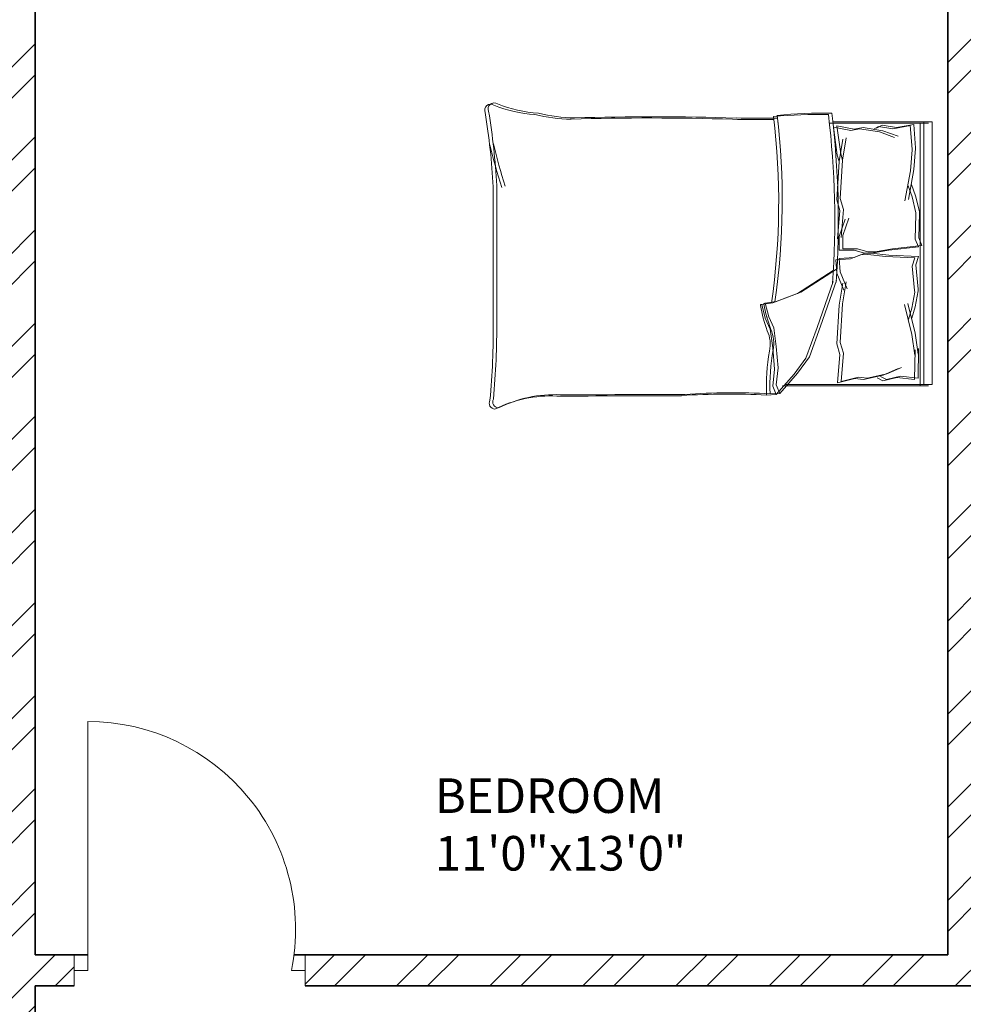
# Model space of a CAD drawing. Units: inches. Extents: x 1962 to 2771, y 1245 to 2660.
# Tile 111 of 114: x 2374 to 2510, y 2304 to 2447. Entities that reach past the tile are written whole.
import ezdxf

# ---------------------------------------------------------------- set-up
doc = ezdxf.new("R2010")
doc.units = ezdxf.units.IN
for name, color, linetype, lineweight in [('A-ANNO-DIMS', 2, 'Continuous', 18), ('A-AREA-IDEN', 7, 'Continuous', 18), ('A-DOOR', 3, 'Continuous', 18), ('A-FURN', 8, 'Continuous', 13), ('A-WALL', 7, 'Continuous', 35), ('A-WALL-PATT', 252, 'Continuous', 13)]:
    doc.layers.add(name, color=color, linetype=linetype, lineweight=lineweight)
doc.styles.get("Standard").update_dxf_attribs({"font": 'arial.ttf'})
doc.dimstyles.get("Standard").update_dxf_attribs({"dimtxt": 0.18, "dimasz": 0.18, "dimexe": 0.18, "dimexo": 0.0625, "dimgap": 0.09, "dimtad": 0, "dimtih": 1, "dimtoh": 1, "dimdec": 4, "dimzin": 0, "dimdsep": 46, "dimtxsty": 'Standard', "dimcen": 0.09, "dimadec": 0, "dimazin": 0, "dimtfac": 1, "dimtdec": 4, "dimtofl": 0, "dimtmove": 0, "dimatfit": 3, "dimfxl": 1, "dimtolj": 1, "dimtzin": 0, "dimarcsym": 0})

# ---------------------------------------------------------------- blocks, each defined once
blk = doc.blocks.new('BED-PLAN')
for p, q in [((22.05, 42.03), (19.47, 39.08)), ((22.05, 42.02), (19.47, 39.08)), ((22.56, 42.21), (19.98, 39.26)), ((22.56, 42.21), (19.98, 39.26)), ((23.44, 42.09), (22.05, 42.03, 3.08)), ((23.44, 42.09), (22.05, 42.02, 3.08)), ((22.55, 40.8), (22.05, 42.03)), ((22.55, 40.8), (22.05, 42.02)), ((23.95, 42.27), (22.56, 42.21, 3.08)), ((23.95, 42.27), (22.56, 42.21, 3.08)), ((23.06, 40.98), (22.56, 42.21)), ((23.06, 40.98), (22.56, 42.21)), ((0, 40.75), (21.15, 40.75)), ((0, 40.75), (21.15, 40.75)), ((0, 2.76), (0, 40.75)), ((0.51, 40.93), (21.66, 40.93)), ((0.51, 40.93), (21.66, 40.93)), ((1.22, 2.76), (1.22, 40.75)), ((1.22, 2.76), (1.22, 40.75)), ((1.73, 2.95), (1.73, 40.93)), ((1.73, 2.95), (1.73, 40.93)), ((2.54, 40.02), (2.46, 35.72)), ((2.54, 40.02), (2.46, 35.72)), ((2.54, 40.02), (5.09, 39.72)), ((2.54, 40.02), (5.09, 39.72)), ((4.58, 39.53), (6.63, 40.01)), ((4.58, 39.53), (6.63, 40.01)), ((5.09, 39.72), (7.14, 40.19)), ((5.09, 39.72), (7.14, 40.19)), ((6.63, 40.01), (7.46, 39.6)), ((6.63, 40.01), (7.46, 39.6)), ((9.91, 40.02), (7.07, 39.38)), ((9.91, 40.02), (7.07, 39.38)), ((7.14, 40.19), (7.97, 39.78)), ((7.14, 40.19), (7.97, 39.78)), ((11.19, 39.87), (9.91, 40.02)), ((11.19, 39.87), (9.91, 40.02)), ((13.17, 40.3), (10.68, 39.68)), ((13.17, 40.3), (10.68, 39.68)), ((13.68, 40.48), (11.19, 39.87)), ((13.68, 40.48), (11.19, 39.87)), ((12.85, 36.22), (13.17, 40.3)), ((12.85, 36.22), (13.17, 40.3)), ((13.36, 36.4), (13.68, 40.48)), ((13.36, 36.4), (13.68, 40.48)), ((22.3, 38.34), (22.55, 40.8)), ((22.3, 38.34), (22.55, 40.8)), ((22.81, 38.52), (23.06, 40.98)), ((22.81, 38.52), (23.06, 40.98)), ((2.03, 39.83), (1.96, 35.54)), ((2.03, 39.83), (1.96, 35.54)), ((2.03, 39.83), (4.58, 39.53)), ((2.03, 39.83), (4.58, 39.53)), ((6.56, 39.2), (4.43, 38.26)), ((6.56, 39.2), (4.43, 38.26)), ((7.07, 39.38), (4.94, 38.44)), ((7.07, 39.38), (4.94, 38.44)), ((9.4, 39.83), (6.56, 39.2)), ((9.4, 39.83), (6.56, 39.2)), ((10.68, 39.68), (9.4, 39.83)), ((10.68, 39.68), (9.4, 39.83)), ((19.47, 39.08), (17.75, 36.74)), ((19.47, 39.08), (17.75, 36.74)), ((19.98, 39.26), (18.26, 36.92)), ((19.98, 39.26), (18.26, 36.92)), ((23.06, 35.45), (22.81, 38.52)), ((23.06, 35.44), (22.81, 38.52)), ((22.55, 35.26), (22.3, 38.34)), ((22.55, 35.26), (22.3, 38.34)), ((1.96, 35.54), (2.02, 36.34)), ((1.96, 35.54), (2.02, 36.34)), ((2.02, 36.34), (2.44, 33.32)), ((2.02, 36.34), (2.44, 33.32)), ((2.46, 35.72), (2.53, 36.52)), ((2.46, 35.72), (2.53, 36.52)), ((2.53, 36.52), (2.95, 33.5)), ((2.53, 36.52), (2.95, 33.5)), ((13.3, 34.66), (12.85, 36.22)), ((13.3, 34.66), (12.85, 36.22)), ((13.8, 34.84), (13.36, 36.4)), ((13.8, 34.84), (13.36, 36.4)), ((17.75, 36.74), (16.15, 32.31)), ((17.75, 36.74), (16.15, 32.31)), ((18.26, 36.92), (16.66, 32.49)), ((18.26, 36.92), (16.66, 32.49)), ((12.95, 29.09), (13.3, 34.66)), ((12.95, 29.09), (13.3, 34.66)), ((13.46, 29.27), (13.8, 34.84)), ((13.46, 29.27), (13.8, 34.84)), ((22.92, 32.56), (22.55, 35.26)), ((22.92, 32.55), (22.55, 35.26)), ((23.42, 32.74), (23.06, 35.45)), ((23.42, 32.74), (23.06, 35.44)), ((2.44, 33.32), (3.52, 29.01)), ((2.44, 33.32), (3.52, 29.01)), ((2.95, 33.5), (4.02, 29.19)), ((2.95, 33.5), (4.02, 29.19)), ((3.43, 31.34), (2.96, 29.7)), ((3.43, 31.34), (2.96, 29.7)), ((16.15, 32.31), (13.82, 25.68)), ((16.15, 32.31), (13.82, 25.68)), ((16.66, 32.49), (14.33, 25.86)), ((16.66, 32.49), (14.33, 25.86)), ((23.65, 30.95), (22.92, 32.56)), ((23.65, 30.95), (22.92, 32.55)), ((24.16, 31.14), (23.42, 32.74)), ((24.16, 31.14), (23.42, 32.74)), ((62.99, 11.98), (62.99, 31.54)), ((62.99, 11.97), (62.99, 31.54)), ((63.5, 12.16), (63.5, 31.72)), ((63.5, 12.16), (63.5, 31.72)), ((2.92, 31.16), (2.45, 29.52)), ((2.92, 31.16), (2.45, 29.52)), ((24.15, 28.99), (23.65, 30.95)), ((24.15, 28.98), (23.65, 30.95)), ((24.65, 29.17), (24.16, 31.14)), ((24.65, 29.17), (24.16, 31.14)), ((2.45, 29.52), (2.02, 27.19)), ((2.45, 29.52), (2.02, 27.19)), ((2.96, 29.7), (2.52, 27.37)), ((2.96, 29.7), (2.52, 27.37)), ((12.42, 25.89), (12.95, 29.09)), ((12.42, 25.89), (12.95, 29.09)), ((12.93, 26.07), (13.46, 29.27)), ((12.93, 26.07), (13.46, 29.27)), ((18.98, 27.38), (22.55, 28.74)), ((18.98, 27.38), (22.55, 28.74)), ((19.49, 27.57), (23.06, 28.92)), ((19.49, 27.57), (23.06, 28.92)), ((22.55, 28.74), (24.15, 28.99)), ((22.55, 28.74), (24.15, 28.98)), ((23.06, 28.92), (24.65, 29.17)), ((23.06, 28.92), (24.65, 29.17)), ((2.02, 27.19), (2.03, 26.94)), ((2.02, 27.19), (2.03, 26.93)), ((2.52, 27.37), (2.54, 27.12)), ((2.52, 27.37), (2.54, 27.12)), ((2.54, 27.12), (2.88, 23.6)), ((2.54, 27.12), (2.88, 23.6)), ((13.82, 24.05), (18.98, 27.38)), ((13.82, 24.05), (18.98, 27.38)), ((14.33, 24.24), (19.49, 27.57)), ((14.33, 24.24), (19.49, 27.57)), ((2.03, 26.94), (2.37, 23.42)), ((2.03, 26.93), (2.37, 23.42)), ((13.31, 24.44), (12.28, 26.89)), ((13.31, 24.44), (12.28, 26.88)), ((13.81, 24.63), (12.79, 27.07)), ((13.81, 24.63), (12.79, 27.07)), ((13.43, 22.49), (13.31, 24.44)), ((13.43, 22.49), (13.31, 24.44)), ((13.94, 22.68), (13.81, 24.63)), ((13.94, 22.68), (13.81, 24.63)), ((2.37, 23.42), (1.98, 22.24)), ((2.37, 23.42), (1.98, 22.24)), ((2.88, 23.6), (2.49, 22.42)), ((2.88, 23.6), (2.49, 22.42)), ((1.98, 22.24), (6.25, 22.05)), ((1.98, 22.24), (6.25, 22.05)), ((2.49, 22.42), (6.76, 22.23)), ((2.49, 22.42), (6.76, 22.23)), ((5.74, 21.11), (8.27, 21.57)), ((5.74, 21.11), (8.27, 21.57)), ((6.25, 22.05), (8.81, 21.75)), ((6.25, 22.05), (8.81, 21.75)), ((6.25, 21.3), (8.78, 21.76)), ((6.25, 21.3), (8.78, 21.76)), ((6.76, 22.23), (9.31, 21.93)), ((6.76, 22.23), (9.31, 21.93)), ((8.27, 21.57), (9.3, 21.57)), ((8.27, 21.57), (9.3, 21.57)), ((8.78, 21.76), (9.81, 21.76)), ((8.78, 21.76), (9.81, 21.76)), ((8.81, 21.75), (9.84, 21.81)), ((8.81, 21.75), (9.84, 21.81)), ((9.3, 21.57), (10.8, 21.11)), ((9.3, 21.57), (10.8, 21.11)), ((9.31, 21.93), (10.35, 21.99)), ((9.31, 21.93), (10.35, 21.99)), ((9.81, 21.76), (11.3, 21.3)), ((9.81, 21.76), (11.3, 21.3)), ((9.84, 21.81), (11.3, 22.36)), ((9.84, 21.81), (11.3, 22.36)), ((10.35, 21.99), (11.81, 22.54)), ((10.35, 21.99), (11.81, 22.54)), ((11.3, 22.36), (13.43, 22.49)), ((11.3, 22.36), (13.43, 22.49)), ((11.81, 22.54), (13.94, 22.68)), ((11.81, 22.54), (13.94, 22.68)), ((1.49, 20.65), (5.74, 21.11)), ((1.49, 20.65), (5.74, 21.11)), ((1.95, 19.51), (1.49, 20.65)), ((1.95, 19.51), (1.49, 20.65)), ((1.99, 20.84), (6.25, 21.3)), ((1.99, 20.84), (6.25, 21.3)), ((2.45, 19.69), (1.99, 20.84)), ((2.45, 19.69), (1.99, 20.84)), ((10.8, 21.11), (12.93, 21.11)), ((10.8, 21.11), (12.93, 21.11)), ((11.3, 21.3), (13.44, 21.3)), ((11.3, 21.3), (13.44, 21.3)), ((12.93, 21.11), (12.93, 19.16)), ((12.93, 21.11), (12.93, 19.16)), ((13.44, 21.3), (13.44, 19.34)), ((13.44, 21.3), (13.44, 19.34)), ((1.83, 15.97), (1.95, 19.51)), ((1.83, 15.97), (1.95, 19.51)), ((2.34, 16.15), (2.45, 19.69)), ((2.34, 16.15), (2.45, 19.69)), ((12.93, 19.16), (12.06, 16.66)), ((12.93, 19.16), (12.06, 16.66)), ((13.44, 19.34), (12.57, 16.84)), ((13.44, 19.34), (12.57, 16.84)), ((12.85, 15.41), (13.17, 19.49)), ((12.85, 15.41), (13.17, 19.49)), ((13.36, 15.59), (13.68, 19.67)), ((13.36, 15.59), (13.68, 19.67)), ((1.83, 15.72), (1.83, 15.97)), ((1.83, 15.72), (1.83, 15.97)), ((2.41, 13.42), (1.83, 15.72)), ((2.41, 13.42), (1.83, 15.72)), ((2.34, 15.9), (2.34, 16.15)), ((2.34, 15.9), (2.34, 16.15)), ((2.91, 13.6), (2.34, 15.9)), ((2.91, 13.6), (2.34, 15.9)), ((13.3, 13.85), (12.85, 15.41)), ((13.3, 13.85), (12.85, 15.41)), ((13.8, 14.03), (13.36, 15.59)), ((13.8, 14.03), (13.36, 15.59)), ((2.98, 11.81), (2.41, 13.42)), ((2.98, 11.81), (2.41, 13.42)), ((2.64, 9.63), (3.44, 13.99)), ((2.64, 9.63), (3.44, 13.99)), ((3.49, 11.99), (2.91, 13.6)), ((3.49, 11.99), (2.91, 13.6)), ((3.14, 9.81), (3.95, 14.17)), ((3.14, 9.81), (3.95, 14.17)), ((12.95, 8.28), (13.3, 13.85)), ((12.95, 8.28), (13.3, 13.85)), ((13.46, 8.46), (13.8, 14.03)), ((13.46, 8.46), (13.8, 14.03)), ((2.41, 6.59), (2.64, 9.63)), ((2.41, 6.59), (2.64, 9.63)), ((2.91, 6.77), (3.14, 9.81)), ((2.91, 6.77), (3.14, 9.81)), ((12.42, 5.07), (12.95, 8.28)), ((12.42, 5.07), (12.95, 8.28)), ((12.93, 5.26), (13.46, 8.46)), ((12.93, 5.26), (13.46, 8.46)), ((12.95, 8.28), (13.21, 7.38)), ((12.95, 8.28), (13.21, 7.38)), ((13.21, 7.38), (13.78, 3.33)), ((13.21, 7.38), (13.78, 3.33)), ((13.46, 8.46), (13.72, 7.56)), ((13.46, 8.46), (13.72, 7.56)), ((13.72, 7.56), (14.29, 3.51)), ((13.72, 7.56), (14.29, 3.51)), ((2.39, 6.5), (2.41, 6.59)), ((2.39, 6.5), (2.41, 6.59)), ((2.65, 3.1), (2.39, 6.5)), ((2.65, 3.1), (2.39, 6.5)), ((2.9, 6.68), (2.91, 6.77)), ((2.9, 6.68), (2.91, 6.77)), ((3.16, 3.28), (2.9, 6.68)), ((3.16, 3.28), (2.9, 6.68)), ((7.12, 4.02), (4.93, 4.82)), ((7.12, 4.02), (4.93, 4.82)), ((7.63, 4.2), (5.44, 5)), ((7.63, 4.2), (5.44, 5)), ((14.9, 2.95), (0.51, 2.95)), ((14.9, 2.95), (0.51, 2.95)), ((2.64, 3.1), (5.16, 3.56)), ((2.64, 3.1), (5.16, 3.56)), ((3.14, 3.28), (5.67, 3.74)), ((3.14, 3.28), (5.67, 3.74)), ((5.16, 3.56), (7.23, 3.21)), ((5.16, 3.56), (7.23, 3.21)), ((5.67, 3.74), (7.74, 3.39)), ((5.67, 3.74), (7.74, 3.39)), ((9.99, 3.56), (7.12, 4.02)), ((9.99, 3.56), (7.12, 4.02)), ((7.23, 3.21), (8.04, 3.67)), ((7.23, 3.21), (8.04, 3.67)), ((10.5, 3.74), (7.63, 4.2)), ((10.5, 3.74), (7.63, 4.2)), ((7.74, 3.39), (8.55, 3.85)), ((7.74, 3.39), (8.55, 3.85)), ((11.26, 3.79), (9.99, 3.56)), ((11.26, 3.79), (9.99, 3.56)), ((11.76, 3.97), (10.5, 3.74)), ((11.76, 3.97), (10.5, 3.74)), ((13.78, 3.33), (11.26, 3.79)), ((13.78, 3.33), (11.26, 3.79)), ((14.29, 3.51), (11.76, 3.97)), ((14.29, 3.51), (11.76, 3.97)), ((14.4, 2.76), (0, 2.76)), ((14.4, 2.76), (0, 2.76))]:
    blk.add_line(p, q)
for centre, radius, start, end in [((55.09, 60.72), 18.33, 267.4714, 296.4681), ((55.09, 60.72), 18.33, 267.4714, 296.4681), ((63.2, 43.43), 0.876, 332.6588, 86.02), ((63.2, 43.43), 0.876, 332.6588, 86.02), ((54.58, 60.54), 18.33, 267.4714, 296.4681), ((54.58, 60.54), 18.33, 267.4714, 296.4681), ((62.69, 43.25), 0.876, 332.6588, 86.02), ((62.69, 43.25), 0.876, 332.6588, 86.02), ((168.74, 32.71), 105.75, 174.4998, 180.6351), ((168.74, 32.71), 105.75, 174.4998, 180.6351), ((169.24, 32.89), 105.75, 174.4998, 180.6351), ((169.24, 32.89), 105.75, 174.4998, 180.6351), ((-5.29, 40.8), 28.76, 349.8763, 2.5657), ((-5.29, 40.8), 28.76, 349.8763, 2.5657), ((28.87, 144.88), 102.94, 266.9791, 273.8365), ((28.87, 144.88), 102.94, 266.9791, 273.8365), ((-4.78, 40.98), 28.76, 349.8763, 2.5657), ((-4.78, 40.98), 28.76, 349.8763, 2.5657), ((29.37, 145.06), 102.94, 266.9791, 273.8365), ((29.37, 145.06), 102.94, 266.9791, 273.8365), ((53.91, -3583.94), 3626.16, 90.00217, 90.28689), ((53.91, -3583.94), 3626.16, 90.00217, 90.28689), ((54.42, -3583.75), 3626.16, 90.00217, 90.28689), ((54.42, -3583.75), 3626.16, 90.00217, 90.28689), ((27.87, 34.77), 4.95, 168.6608, 203.7384), ((27.87, 34.77), 4.95, 168.6608, 203.7384), ((28.38, 34.95), 4.95, 168.6608, 203.7384), ((28.38, 34.95), 4.95, 168.6608, 203.7384), ((1.18, 24.77), 23.57, 10.6617, 19.8806), ((1.18, 24.76), 23.57, 10.6617, 19.8806), ((1.69, 24.95), 23.57, 10.6617, 19.8806), ((1.69, 24.95), 23.57, 10.6617, 19.8806), ((124.25, 14.12), 102.56, 171.7845, 186.9006), ((124.25, 14.11), 102.56, 171.7845, 186.9006), ((124.76, 14.3), 102.56, 171.7845, 186.9006), ((124.76, 14.3), 102.56, 171.7845, 186.9006), ((24.2, 29.12), 0.147, 250.2464, 1.1377), ((24.2, 29.12), 0.147, 250.2464, 1.1377), ((24.7, 29.3), 0.147, 250.2464, 1.1377), ((24.7, 29.3), 0.147, 250.2464, 1.1377), ((144.71, 16.98), 131.13, 176.0865, 186.7821), ((144.71, 16.98), 131.13, 176.0865, 186.7821), ((145.22, 17.16), 131.13, 176.0865, 186.7821), ((145.22, 17.16), 131.13, 176.0865, 186.7821), ((-18.85, -13.69), 84.62, 13.3832, 17.7053), ((-18.85, -13.69), 84.62, 13.3832, 17.7053), ((-18.34, -13.51), 84.62, 13.3832, 17.7053), ((-18.34, -13.51), 84.62, 13.3832, 17.7053), ((159.64, 17.03), 96.78, 182.9958, 189.4091), ((159.64, 17.03), 96.78, 182.9958, 189.4091), ((160.15, 17.21), 96.78, 182.9958, 189.4091), ((160.15, 17.21), 96.78, 182.9958, 189.4091), ((15.97, 67.7), 66.22, 268.7218, 275.604), ((15.97, 67.7), 66.22, 268.7218, 275.604), ((16.48, 67.88), 66.22, 268.7218, 275.604), ((16.48, 67.88), 66.22, 268.7218, 275.604), ((24.78, -132.99), 135.22, 88.4762, 91.0082), ((24.78, -132.99), 135.22, 88.4762, 91.0082), ((25.29, -132.81), 135.22, 88.4762, 91.0082), ((25.29, -132.81), 135.22, 88.4762, 91.0082), ((40.23, 385.38), 383.38, 268.2277, 271.7185), ((40.23, 385.38), 383.38, 268.2277, 271.7185), ((40.74, 385.56), 383.38, 268.2277, 271.7185), ((40.74, 385.56), 383.38, 268.2277, 271.7185), ((51.28, -21.38), 23.56, 76.0648, 88.9113), ((51.28, -21.38), 23.56, 76.0648, 88.9113), ((51.79, -21.2), 23.56, 76.0648, 88.9113), ((51.79, -21.2), 23.56, 76.0648, 88.9113), ((55.86, -17.22), 18.73, 67.9751, 86.652), ((55.86, -17.22), 18.73, 67.9751, 86.652), ((56.37, -17.03), 18.73, 67.9751, 86.652), ((56.37, -17.03), 18.73, 67.9751, 86.652), ((63.37, 0.87), 0.866, 236.1736, 23.4781), ((63.37, 0.87), 0.866, 236.1736, 23.4781), ((63.87, 1.05), 0.866, 236.1736, 23.4781), ((63.87, 1.05), 0.866, 236.1736, 23.4781)]:
    blk.add_arc(centre, radius, start, end)
blk = doc.blocks.new('*D40')
at = {"layer": 'A-ANNO-DIMS', "color": 0, "lineweight": -2, "transparency": 16777216}
for p, q in [((2072.02, 2033.91), (2072.02, 2583.47)), ((2072.2, 2583.29), (2366.02, 2583.29)), ((2660.63, 2583.29), (2366.81, 2583.29)), ((2660.81, 2524.41), (2660.81, 2583.47))]:
    blk.add_line(p, q, dxfattribs=at)
at = {"layer": 'A-ANNO-DIMS', "color": 0, "transparency": 16777216}
for points in [[(2072.2, 2583.32), (2072.2, 2583.26), (2072.02, 2583.29)], [(2660.63, 2583.32), (2660.63, 2583.26), (2660.81, 2583.29)]]:
    blk.add_solid(points, dxfattribs=at)
at = {"layer": 'Defpoints', "color": 0, "transparency": 16777216}
for p in [(2660.81, 2583.29), (2660.81, 2524.34), (2072.02, 2033.84)]:
    blk.add_point(p, dxfattribs=at)
at = {"layer": 'A-ANNO-DIMS', "color": 0, "transparency": 16777216, "insert": (2366.41, 2583.29), "char_height": 0.18, "attachment_point": 5}
blk.add_mtext('\\A1;588.8', dxfattribs=at)

msp = doc.modelspace()

# ---------------------------------------------------------------- hatches: boundary and pattern name
at = {"layer": 'A-WALL-PATT'}
h = msp.add_hatch(dxfattribs=at)
h.set_pattern_fill('ANSI32', color=256)
h.paths.add_polyline_path([(2090.8074, 2467.3437), (2141.6481, 2467.3437), (2141.6481, 2469.5937), (2141.6481, 2471.8437), (2086.3074, 2471.8437), (2086.3074, 2422.5333), (2090.8074, 2422.5333)])
h.paths.add_polyline_path([(2282.7664, 2471.8437), (2204.8982, 2471.8437), (2204.8982, 2467.3437), (2234.8074, 2467.3437), (2234.8074, 2311.3437), (2228.7492, 2311.3437), (2228.7492, 2306.8437), (2234.8074, 2306.8437), (2331.9227, 2306.8437), (2331.9227, 2309.0937), (2331.9227, 2311.3437), (2239.3074, 2311.3437), (2239.3074, 2467.3437), (2282.7664, 2467.3437), (2282.7664, 2469.5937)])
h.paths.add_polyline_path([(2471.4531, 2519.8437), (2552.011, 2519.8437), (2564.3996, 2519.8437), (2564.3996, 2511.1389), (2568.8996, 2511.1389), (2568.8996, 2524.3437), (2466.9531, 2524.3437), (2466.9531, 2471.8437), (2450.0749, 2471.8437), (2446.4672, 2471.8437), (2446.4672, 2467.3437), (2450.0749, 2467.3437), (2475.9988, 2467.3437), (2475.9988, 2469.5937), (2475.9988, 2471.8437), (2471.4531, 2471.8437)])
h.paths.add_polyline_path([(2575.2231, 2469.5937), (2575.2231, 2471.8437), (2568.8996, 2471.8437), (2568.8996, 2487.1389), (2564.3996, 2487.1389), (2564.3996, 2471.8437), (2556.511, 2471.8437), (2499.2904, 2471.8437), (2499.2904, 2467.3437), (2507.8074, 2467.3437), (2507.8074, 2311.3437), (2414.863, 2311.3437), (2414.863, 2306.8437), (2512.3074, 2306.8437), (2517.0114, 2306.8437), (2517.0114, 2309.0937), (2517.0114, 2311.3437), (2512.3074, 2311.3437), (2512.3074, 2467.3437), (2575.2231, 2467.3437)])
h.paths.add_polyline_path([(2660.8074, 2471.8437), (2600.9602, 2471.8437), (2600.9602, 2467.3437), (2656.3074, 2467.3437), (2656.3074, 2432.5704), (2660.8074, 2432.5704)])
h.paths.add_polyline_path([(2660.8074, 2372.5704), (2656.3074, 2372.5704), (2656.3074, 2311.3437), (2600.276, 2311.3437), (2600.276, 2309.0937), (2600.276, 2306.8437), (2656.3074, 2306.8437), (2656.3074, 2296.2593), (2660.8074, 2296.2593)])
h.paths.add_polyline_path([(2572.3074, 2306.8437), (2577.1385, 2306.8437), (2577.1385, 2311.3437), (2551.082, 2311.3437), (2551.082, 2306.8437), (2567.8074, 2306.8437), (2567.8074, 2258.8437), (2540.0574, 2258.8437), (2540.0574, 2256.5937), (2540.0574, 2254.3437), (2567.8074, 2254.3437), (2656.3074, 2254.3437), (2656.3074, 2236.9085), (2660.8074, 2236.9085), (2660.8074, 2272.2593), (2656.3074, 2272.2593), (2656.3074, 2258.8437), (2572.3074, 2258.8437)])
h.paths.add_polyline_path([(2512.3074, 2254.3437), (2518.8716, 2254.3437), (2518.8716, 2256.5937), (2518.8716, 2258.8437), (2507.8074, 2258.8437), (2507.8074, 2177.8437), (2567.8074, 2177.8437), (2567.8074, 2172.9628), (2572.3074, 2172.9628), (2572.3074, 2177.8437), (2656.3074, 2177.8437), (2656.3074, 2166.4846), (2660.8074, 2166.4846), (2660.8074, 2200.9085), (2656.3074, 2200.9085), (2656.3074, 2182.3437), (2512.3074, 2182.3437)])
h.paths.add_polyline_path([(2656.3074, 2129.8437), (2572.3074, 2129.8437), (2572.3074, 2150.3044), (2570.0574, 2150.3044), (2567.8074, 2150.3044), (2567.8074, 2129.8437), (2507.8074, 2129.8437), (2507.8074, 2116.3027), (2510.0574, 2116.3027), (2512.3074, 2116.3027), (2512.3074, 2125.3437), (2567.8074, 2125.3437), (2572.3074, 2125.3437), (2656.3074, 2125.3437)])
h.paths.add_polyline_path([(2090.8074, 2362.5333), (2086.3074, 2362.5333), (2086.3074, 2298.6242), (2090.8074, 2298.6242), (2090.8074, 2306.8437), (2174.8074, 2306.8437), (2174.8074, 2286.4178), (2179.3074, 2286.4178), (2179.3074, 2306.8437), (2192.8641, 2306.8437), (2192.8641, 2309.0937), (2192.8641, 2311.3437), (2090.8074, 2311.3437)])
h.paths.add_polyline_path([(2209.156, 2258.8437), (2179.3074, 2258.8437), (2179.3074, 2263.2236), (2177.0574, 2263.2236), (2174.8074, 2263.2236), (2174.8074, 2258.8437), (2090.8074, 2258.8437), (2090.8074, 2274.6242), (2086.3074, 2274.6242), (2086.3074, 2238.2967), (2088.5574, 2238.2967), (2090.8074, 2238.2967), (2090.8074, 2254.3437), (2209.156, 2254.3437)])
h.paths.add_polyline_path([(2090.8074, 2177.8437), (2234.8074, 2177.8437), (2234.8074, 2173.1428), (2239.3074, 2173.1428), (2239.3074, 2258.8437), (2230.8442, 2258.8437), (2230.8442, 2256.5937), (2230.8442, 2254.3437), (2234.8074, 2254.3437), (2234.8074, 2182.3437), (2090.8074, 2182.3437), (2090.8074, 2202.2967), (2086.3074, 2202.2967), (2086.3074, 2140.0389), (2090.8074, 2140.0389)])
h.paths.add_polyline_path([(2090.8074, 2080.0389), (2086.3074, 2080.0389), (2086.3074, 2033.8437), (2090.8074, 2033.8437)], flags=17)
h.paths.add_polyline_path([(2244.9405, 2033.8437), (2239.3074, 2033.8437), (2239.3074, 2142.0665), (2237.2592, 2142.0665), (2234.8074, 2142.0665), (2234.8074, 2033.8437), (2090.8074, 2033.8437), (2076.5204, 2033.8437), (2072.0204, 2033.8437), (2072.0204, 2000.4493), (2076.5204, 2000.4493), (2076.5204, 2029.3437), (2090.8074, 2029.3437), (2244.9405, 2029.3437), (2244.9405, 2031.5937)])
h.paths.add_polyline_path([(2234.8074, 1933.3437), (2076.5204, 1933.3437), (2076.5204, 1952.4493), (2074.2704, 1952.4493), (2072.0204, 1952.4493), (2072.0204, 1933.3437), (2072.0204, 1928.8437), (2234.8074, 1928.8437)])
h.paths.add_polyline_path([(2090.8074, 1928.8437), (2086.3074, 1928.8437), (2086.3074, 1906.5013), (2090.8074, 1906.5013)])
h.paths.add_polyline_path([(2090.8074, 1846.5013), (2086.3074, 1846.5013), (2086.3074, 1769.9917), (2088.5574, 1769.9917), (2090.8074, 1769.9917), (2090.8074, 1780.3437), (2234.8074, 1780.3437), (2234.8074, 1708.3437), (2230.3764, 1708.3437), (2230.3764, 1703.8437), (2239.3074, 1703.8437), (2239.3074, 1792.6669), (2237.0574, 1792.6669), (2234.8074, 1792.6669), (2234.8074, 1784.8437), (2090.8074, 1784.8437)])
h.paths.add_polyline_path([(2239.3074, 1928.8437), (2244.9405, 1928.8437), (2244.9405, 1931.0937), (2244.9405, 1933.3437), (2234.8074, 1933.3437), (2234.8074, 1928.8437), (2234.8074, 1825.5949), (2239.3074, 1825.5949)])
h.paths.add_polyline_path([(2148.0425, 1649.0937), (2148.0425, 1651.3437), (2090.8074, 1651.3437), (2090.8074, 1646.8437), (2148.0425, 1646.8437)], flags=0)
h.paths.add_polyline_path([(2207.5601, 1708.3437), (2090.8074, 1708.3437), (2090.8074, 1703.8437), (2174.8074, 1703.8437), (2174.8074, 1651.3437), (2170.4457, 1651.3437), (2170.4457, 1646.8437), (2195.9924, 1646.8437), (2195.9924, 1649.0937), (2195.9924, 1651.3437), (2179.3074, 1651.3437), (2179.3074, 1703.8437), (2207.5601, 1703.8437), (2207.5601, 1706.0937)])
h.paths.add_polyline_path([(2090.8074, 1733.9917), (2086.3074, 1733.9917), (2086.3074, 1696.1032), (2088.5574, 1696.1032), (2090.8074, 1696.1032)])
h.paths.add_polyline_path([(2090.8074, 1672.1032), (2086.3074, 1672.1032), (2086.3074, 1600.3335), (2090.8074, 1600.3335)])
h.paths.add_polyline_path([(2090.8074, 1540.3335), (2086.3074, 1540.3335), (2086.3074, 1486.3437), (2139.6766, 1486.3437), (2139.6766, 1490.8437), (2090.8074, 1490.8437)])
h.paths.add_polyline_path([(2302.3876, 1490.8437), (2239.3074, 1490.8437), (2239.3074, 1646.8437), (2335.9994, 1646.8437), (2335.9994, 1651.3437), (2229.884, 1651.3437), (2229.884, 1646.8437), (2234.8074, 1646.8437), (2234.8074, 1490.8437), (2202.7103, 1490.8437), (2202.7103, 1488.5937), (2202.7103, 1486.3437), (2275.0699, 1486.3437), (2275.0699, 1475.772), (2279.5699, 1475.772), (2279.5699, 1486.3437), (2302.3876, 1486.3437)])
h.paths.add_polyline_path([(2279.5699, 1451.772), (2275.0699, 1451.772), (2275.0699, 1438.3437), (2174.8074, 1438.3437), (2174.8074, 1486.3437), (2179.7922, 1486.3437), (2179.7922, 1490.8437), (2163.3585, 1490.8437), (2163.3585, 1488.5937), (2163.3585, 1486.3437), (2170.3074, 1486.3437), (2170.3074, 1433.8437), (2279.5699, 1433.8437)])
h.paths.add_polyline_path([(2427.2363, 1490.8437), (2375.8074, 1490.8437), (2375.8074, 1646.8437), (2381.6401, 1646.8437), (2381.6401, 1651.3437), (2365.887, 1651.3437), (2365.887, 1649.0937), (2365.887, 1646.8437), (2371.3074, 1646.8437), (2371.3074, 1490.8437), (2327.5627, 1490.8437), (2327.5627, 1488.5937), (2327.5627, 1486.3437), (2371.3074, 1486.3437), (2371.3074, 1433.8437), (2375.8074, 1433.8437), (2375.8074, 1486.3437), (2427.2363, 1486.3437)])
h.paths.add_polyline_path([(2512.3074, 1646.8437), (2519.4351, 1646.8437), (2519.4351, 1649.0937), (2519.4351, 1651.3437), (2507.8074, 1651.3437), (2416.0063, 1651.3437), (2416.0063, 1649.0937), (2416.0063, 1646.8437), (2507.8074, 1646.8437), (2507.8074, 1490.8437), (2497.0532, 1490.8437), (2497.0532, 1488.5937), (2497.0532, 1486.3437), (2574.9344, 1486.3437), (2574.9344, 1476.0181), (2579.4344, 1476.0181), (2579.4344, 1486.3437), (2584.4872, 1486.3437), (2584.3074, 1490.8437), (2512.3074, 1490.8437)])
h.paths.add_polyline_path([(2470.5091, 1486.3437), (2473.9767, 1486.3437), (2473.9767, 1490.8437), (2449.6605, 1490.8437), (2449.6605, 1488.5937), (2449.6605, 1486.3437), (2466.0091, 1486.3437), (2466.0091, 1433.8437), (2470.5091, 1433.8437), (2579.4344, 1433.8437), (2579.4344, 1452.0181), (2574.9344, 1452.0181), (2574.9344, 1438.3437), (2554.5091, 1438.3437), (2470.5091, 1438.3437)])
h.paths.add_polyline_path([(2656.3074, 1490.8437), (2611.86, 1490.8437), (2611.86, 1486.3437), (2656.3074, 1486.3437)])
h.paths.add_polyline_path([(2660.8074, 1532.7007), (2658.5574, 1532.7007), (2656.3074, 1532.7007), (2656.3074, 1486.3437), (2660.8074, 1486.3437)])
h.paths.add_polyline_path([(2660.8074, 1664.9663), (2656.3074, 1664.9663), (2656.3074, 1651.3437), (2602.2313, 1651.3437), (2602.2313, 1646.8437), (2656.3074, 1646.8437), (2656.3074, 1592.7007), (2660.8074, 1592.7007)])
h.paths.add_polyline_path([(2660.8074, 1724.5221), (2656.3074, 1724.5221), (2656.3074, 1703.8437), (2542.4725, 1703.8437), (2542.4725, 1699.3437), (2567.8074, 1699.3437), (2567.8074, 1651.3437), (2552.7766, 1651.3437), (2552.7766, 1649.0937), (2552.7766, 1646.8437), (2577.2878, 1646.8437), (2577.2878, 1649.0937), (2577.2878, 1651.3437), (2572.3074, 1651.3437), (2572.3074, 1699.3437), (2656.3074, 1699.3437), (2656.3074, 1688.9663), (2660.8074, 1688.9663)])
h.paths.add_polyline_path([(2660.8074, 1880.6524), (2656.3074, 1880.6524), (2656.3074, 1832.8437), (2512.3074, 1832.8437), (2512.3074, 1837.8959), (2507.8074, 1837.8959), (2507.8074, 1828.3437), (2567.8074, 1828.3437), (2567.8074, 1804.3437), (2572.3074, 1804.3437), (2572.3074, 1828.3437), (2656.3074, 1828.3437), (2656.3074, 1818.6778), (2660.8074, 1818.6778)])
h.paths.add_polyline_path([(2660.8074, 1794.6778), (2656.3074, 1794.6778), (2656.3074, 1780.3437), (2572.3074, 1780.3437), (2572.3074, 1783.0303), (2570.0574, 1783.0303), (2567.8074, 1783.0303), (2567.8074, 1780.3437), (2507.8074, 1780.3437), (2507.8074, 1699.3437), (2517.8858, 1699.3437), (2517.8858, 1701.5937), (2517.8858, 1703.8437), (2512.3074, 1703.8437), (2512.3074, 1775.8437), (2656.3074, 1775.8437), (2656.3074, 1760.5221), (2660.8074, 1760.5221)])
h.paths.add_polyline_path([(2660.8074, 1981.3437), (2660.8074, 2020.2808), (2658.5574, 2020.2808), (2656.3074, 2020.2808), (2656.3074, 1981.3437), (2512.3074, 1981.3437), (2512.3074, 2086.6996), (2507.8074, 2086.6996), (2507.8074, 1981.3437), (2375.8074, 1981.3437), (2375.8074, 1986.8505), (2373.5574, 1986.8505), (2371.3074, 1986.8505), (2371.3074, 1973.2607), (2375.8074, 1973.2607), (2375.8074, 1976.8437), (2507.8074, 1976.8437), (2507.8074, 1865.4281), (2510.0574, 1865.4281), (2512.3074, 1865.4281), (2512.3074, 1976.8437), (2660.8074, 1976.8437)])
h.paths.add_polyline_path([(2375.8074, 1940.297), (2373.5574, 1940.297), (2371.3074, 1940.297), (2371.3074, 1933.3437), (2278.4434, 1933.3437), (2278.4434, 1928.8437), (2371.3074, 1928.8437), (2371.3074, 1651.3437), (2375.8074, 1651.3437)])
h.paths.add_polyline_path([(2660.8074, 1976.8437), (2656.3074, 1976.8437), (2656.3074, 1940.6524), (2660.8074, 1940.6524)], flags=17)
h.paths.add_polyline_path([(2660.8074, 2142.4846), (2656.3074, 2142.4846), (2656.3074, 2080.2808), (2660.8074, 2080.2808)])
h.paths.add_polyline_path([(2381.4189, 2311.3437), (2375.8074, 2311.3437), (2375.8074, 2467.3437), (2424.7242, 2467.3437), (2424.7242, 2469.5937), (2424.7242, 2471.8437), (2375.8074, 2471.8437), (2375.8074, 2524.3437), (2371.3074, 2524.3437), (2371.3074, 2471.8437), (2307.2097, 2471.8437), (2307.2097, 2467.3437), (2371.3074, 2467.3437), (2371.3074, 2311.3437), (2366.8901, 2311.3437), (2366.8901, 2306.8437), (2371.3074, 2306.8437), (2371.3074, 2033.8437), (2279.6589, 2033.8437), (2279.6589, 2029.3437), (2371.3074, 2029.3437), (2371.3074, 2014.2598), (2375.8074, 2014.2598), (2375.8074, 2306.8437), (2381.4189, 2306.8437)])
h.paths.add_polyline_path([(2263.3074, 2524.3437), (2170.3074, 2524.3437), (2170.3074, 2519.8437), (2170.3074, 2471.8437), (2165.0312, 2471.8437), (2165.0312, 2467.3437), (2179.6721, 2467.3437), (2179.6721, 2469.5161), (2179.6721, 2471.8437), (2174.8074, 2471.8437), (2174.8074, 2519.8437), (2258.8074, 2519.8437), (2258.8074, 2511.6436), (2263.3074, 2511.6436)])
h.paths.add_polyline_path([(2245.0232, 1361.4123), (2492.9468, 1361.4123), (2492.9468, 1398.505), (2245.0232, 1398.505)], flags=9)
h.paths.add_polyline_path([(2388.1434, 2086.6936), (2425.0704, 2086.6936), (2425.0704, 2105.3509), (2388.1434, 2105.3509)], flags=9)
h.paths.add_polyline_path([(2404.922, 2242.6744), (2445.7337, 2242.6744), (2445.7337, 2261.3318), (2404.922, 2261.3318)], flags=9)
h.paths.add_polyline_path([(2269.4107, 2156.7935), (2306.3378, 2156.7935), (2306.3378, 2175.4508), (2269.4107, 2175.4508)], flags=9)
h.paths.add_polyline_path([(2269.3277, 2233.4343), (2306.2547, 2233.4343), (2306.2547, 2252.0917), (2269.3277, 2252.0917)], flags=9)
h.paths.add_polyline_path([(2431.6052, 2320.6922), (2470.4456, 2320.6922), (2470.4456, 2339.3495), (2431.6052, 2339.3495)], flags=25)
h.paths.add_polyline_path([(2249.6902, 2315.7608), (2288.5306, 2315.7608), (2288.5306, 2334.4182), (2249.6902, 2334.4182)], flags=25)
h.paths.add_polyline_path([(2096.9301, 2314.3181), (2135.7704, 2314.3181), (2135.7704, 2332.9755), (2096.9301, 2332.9755)], flags=25)
h.paths.add_polyline_path([(2134.3475, 2285.7089), (2161.4655, 2285.7089), (2161.4655, 2304.3662), (2134.3475, 2304.3662)], flags=9)
h.paths.add_polyline_path([(2126.5155, 2209.4076), (2159.9227, 2209.4076), (2159.9227, 2228.065), (2126.5155, 2228.065)], flags=25)
h.paths.add_polyline_path([(2110.5753, 2141.5299), (2149.4157, 2141.5299), (2149.4157, 2160.1872), (2110.5753, 2160.1872)], flags=25)
h.paths.add_polyline_path([(2249.8618, 1968.3317), (2286.3966, 1968.3317), (2286.3966, 1986.989), (2249.8618, 1986.989)], flags=9)
h.paths.add_polyline_path([(2395.9507, 1777.0051), (2436.7624, 1777.0051), (2436.7624, 1795.6625), (2395.9507, 1795.6625)], flags=9)
h.paths.add_polyline_path([(2398.5259, 1888.5651), (2435.0062, 1888.5651), (2435.0062, 1907.2224), (2398.5259, 1907.2224)], flags=25)
h.paths.add_polyline_path([(2259.3506, 1728.3559), (2296.2776, 1728.3559), (2296.2776, 1747.0132), (2259.3506, 1747.0132)], flags=9)
h.paths.add_polyline_path([(2271.3698, 1845.268), (2308.2968, 1845.268), (2308.2968, 1863.9253), (2271.3698, 1863.9253)], flags=9)
h.paths.add_polyline_path([(2120.9355, 1786.3027), (2159.7759, 1786.3027), (2159.7759, 1804.9601), (2120.9355, 1804.9601)], flags=25)
h.paths.add_polyline_path([(2121.3164, 1732.1043), (2154.7236, 1732.1043), (2154.7236, 1750.7616), (2121.3164, 1750.7616)], flags=25)
h.paths.add_polyline_path([(2118.3706, 1678.8997), (2147.5282, 1678.8997), (2147.5282, 1697.557), (2118.3706, 1697.557)], flags=25)
h.paths.add_polyline_path([(2385.9227, 1493.557), (2424.763, 1493.557), (2424.763, 1512.2143), (2385.9227, 1512.2143)], flags=25)
h.paths.add_polyline_path([(2248.7058, 1500.0256), (2287.5462, 1500.0256), (2287.5462, 1518.6829), (2248.7058, 1518.6829)], flags=25)
h.paths.add_polyline_path([(2104.1669, 1617.3771), (2143.0073, 1617.3771), (2143.0073, 1636.0344), (2104.1669, 1636.0344)], flags=9)
h.paths.add_polyline_path([(2096.0714, 1447.8824), (2137.3845, 1447.8824), (2137.3845, 1458.1859), (2096.0714, 1458.1859)], flags=9)
h.paths.add_polyline_path([(2180.6114, 1440.325), (2209.7689, 1440.325), (2209.7689, 1458.9823), (2180.6114, 1458.9823)], flags=25)
h.paths.add_polyline_path([(2316.1698, 1447.9637), (2357.4829, 1447.9637), (2357.4829, 1458.2673), (2316.1698, 1458.2673)], flags=9)
h.paths.add_polyline_path([(2397.6187, 1447.9637), (2438.9318, 1447.9637), (2438.9318, 1458.2673), (2397.6187, 1458.2673)], flags=9)
h.paths.add_polyline_path([(2473.0778, 1439.5953), (2502.2354, 1439.5953), (2502.2354, 1458.2527), (2473.0778, 1458.2527)], flags=25)
h.paths.add_polyline_path([(2589.7027, 1447.8819), (2631.0158, 1447.8819), (2631.0158, 1458.1855), (2589.7027, 1458.1855)], flags=9)
h.paths.add_polyline_path([(2522.4009, 1497.5285), (2561.2413, 1497.5285), (2561.2413, 1516.1859), (2522.4009, 1516.1859)], flags=25)
h.paths.add_polyline_path([(2579.6565, 1671.3482), (2608.8141, 1671.3482), (2608.8141, 1690.0056), (2579.6565, 1690.0056)], flags=25)
h.paths.add_polyline_path([(2544.7038, 1725.5064), (2578.1111, 1725.5064), (2578.1111, 1744.1637), (2544.7038, 1744.1637)], flags=25)
h.paths.add_polyline_path([(2578.1191, 1807.472), (2607.2766, 1807.472), (2607.2766, 1826.1293), (2578.1191, 1826.1293)], flags=25)
h.paths.add_polyline_path([(2595.0614, 1835.1839), (2633.9018, 1835.1839), (2633.9018, 1853.8413), (2595.0614, 1853.8413)], flags=25)
h.paths.add_polyline_path([(2567.0097, 2097.7035), (2605.8501, 2097.7035), (2605.8501, 2116.3609), (2567.0097, 2116.3609)], flags=9)
h.paths.add_polyline_path([(2586.644, 2134.6454), (2615.8015, 2134.6454), (2615.8015, 2153.3027), (2586.644, 2153.3027)], flags=9)
h.paths.add_polyline_path([(2544.6185, 2212.6783), (2578.0258, 2212.6783), (2578.0258, 2231.3356), (2544.6185, 2231.3356)], flags=25)
h.paths.add_polyline_path([(2577.0273, 2256.9023), (2606.1849, 2256.9023), (2606.1849, 2275.5597), (2577.0273, 2275.5597)], flags=24)
h.paths.add_polyline_path([(2605.2683, 2315.2821), (2644.1087, 2315.2821), (2644.1087, 2333.9395), (2605.2683, 2333.9395)], flags=25)
h.paths.add_polyline_path([(2583.1244, 2496.1815), (2624.4375, 2496.1815), (2624.4375, 2506.4851), (2583.1244, 2506.4851)], flags=9)
h.paths.add_polyline_path([(2474.761, 2497.0823), (2503.9185, 2497.0823), (2503.9185, 2515.7397), (2474.761, 2515.7397)], flags=25)
h.paths.add_polyline_path([(2387.5787, 2494.2563), (2428.902, 2494.2563), (2428.902, 2504.5598), (2387.5787, 2504.5598)], flags=9)
h.paths.add_polyline_path([(2300.1657, 2500.1564), (2341.4788, 2500.1564), (2341.4788, 2510.46), (2300.1657, 2510.46)], flags=25)
h.paths.add_polyline_path([(2176.8589, 2497.5843), (2206.0165, 2497.5843), (2206.0165, 2516.2416), (2176.8589, 2516.2416)], flags=25)
h.paths.add_polyline_path([(2097.4668, 2494.9762), (2138.7799, 2494.9762), (2138.7799, 2505.2798), (2097.4668, 2505.2798)], flags=9)

# ---------------------------------------------------------------- linework, layer by layer
at = {"layer": 'A-DOOR'}
for p, q in [((2383.4189, 2309.0937), (2383.4189, 2345.0937)), ((2381.4189, 2306.8437), (2381.4189, 2311.3437)), ((2381.4189, 2311.3437), (2381.4189, 2309.0937)), ((2414.863, 2311.3437), (2414.863, 2306.8437)), ((2381.4189, 2309.0937), (2383.4189, 2309.0937)), ((2414.863, 2309.0937), (2412.863, 2309.0937)), ((2414.863, 2306.8437), (2414.863, 2309.0937))]:
    msp.add_line(p, q, dxfattribs=at)
msp.add_arc((2383.4189, 2315.0527), 30.041, 348.558753, 90, dxfattribs=at)
at = {"layer": 'A-WALL'}
for p, q in [((2375.8074, 2467.3437), (2375.8074, 2311.3437)), ((2507.8074, 2467.3437), (2507.8074, 2311.3437)), ((2375.8074, 2311.3437), (2383.4189, 2311.3437)), ((2413.2301, 2311.3437), (2507.8074, 2311.3437)), ((2375.8074, 2306.8437), (2375.8074, 2014.2598)), ((2375.8074, 2306.8437), (2381.4189, 2306.8437)), ((2414.863, 2306.8437), (2512.3074, 2306.8437))]:
    msp.add_line(p, q, dxfattribs=at)

# ---------------------------------------------------------------- block references
at = {"layer": 'A-FURN', "rotation": 180}
msp.add_blockref('BED-PLAN', (2505.5537, 2434.5988), dxfattribs=at)

# ---------------------------------------------------------------- texts
at = {"layer": 'A-AREA-IDEN', "insert": (2433.6158, 2336.8649), "char_height": 5, "attachment_point": 1}
msp.add_mtext_dynamic_manual_height_columns('BEDROOM\\P11\'0"x13\'0"', width=151.924367, gutter_width=12.5, heights=[0], dxfattribs=at)

# ---------------------------------------------------------------- dimensions: what is measured, and where the dimension line sits
at = {"layer": 'A-ANNO-DIMS'}
dim = msp.add_linear_dim(base=(2660.8074, 2583.2937), p1=(2072.0204, 2033.8437), p2=(2660.8074, 2524.3437), dimstyle='Standard', override={"dimdec": 1, "dimlfac": 1, "dimrnd": 0, "dimzin": 0, "dimdsep": 46, "dimlunit": 2}, dxfattribs=at)
dim.commit()
dim.dimension.update_dxf_attribs({"geometry": '*D40', "text_midpoint": (2366.4139, 2583.2937)})

doc.saveas('drawing.dxf')
